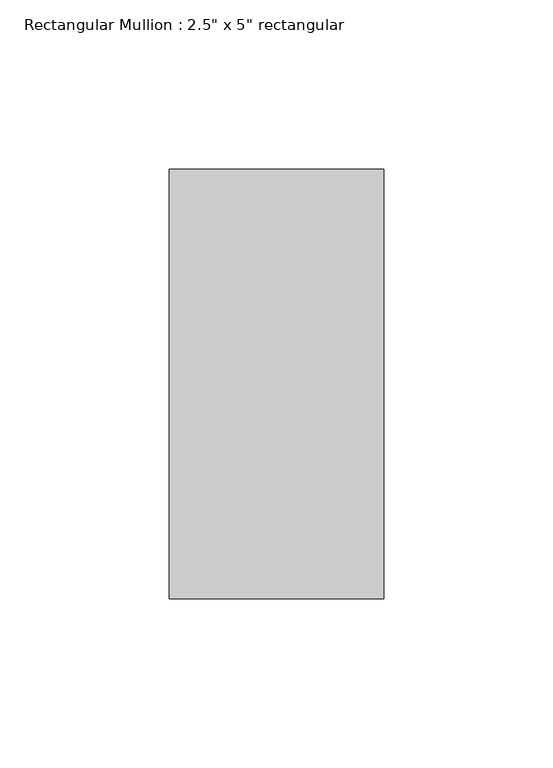
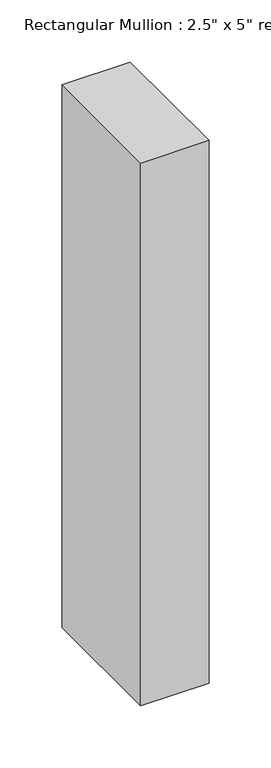
"""IFC4 building model written with IfcOpenShell, lengths in millimetres: member geometry."""

from ifc_helpers import new_model, si_unit, frame, origin, place, context, project, spatial, polyline, outline, extrude, source, transform, mapped, element, save


def member_b281fab0(model_context):
    return source(origin(), model_context, "Body", "SweptSolid", [
        extrude(outline(polyline([(0.0, 63.5), (0.0, -63.5), (-63.5, -63.5), (-63.5, 63.5), (0.0, 63.5)])), frame((0.0, 0.0, -533.4), z_axis=(0.0, 0.0, 1.0), x_axis=(1.0, 0.0, 0.0)), (0.0, 0.0, 1.0), 533.4),
    ])


if __name__ == "__main__":
    model = new_model("IFC4")
    model_context = context("Model", 3, world=origin())
    ifc_project = project(units=[si_unit("LENGTHUNIT", "METRE", prefix="MILLI")], contexts=[model_context])
    site = spatial("IfcSite", under=ifc_project)
    building = spatial("IfcBuilding", under=site)
    placement = place(None, origin())
    member_shape = member_b281fab0(model_context)
    element("IfcMember", 1, ObjectType="Rectangular Mullion : 2.5\" x 5\" rectangular", at=placement, inside=building, context=model_context, shape_type="MappedRepresentation", body=[
        mapped(member_shape, transform((0.0, 0.0, 0.0), x_axis=(1.0, 0.0, 0.0), y_axis=(0.0, 1.0, 0.0), z_axis=(0.0, 0.0, 1.0))),
    ])
    save(model, "model.ifc")

# Revit data of these elements
# Type "Rectangular Mullion : 2.5\" x 5\" rectangular"
#   built-in parameter 1007304 = 0.416667 (stored number, unit not read)
#   built-in parameter 1007301 = 0.104167 (stored number, unit not read)
#   built-in parameter 1007300 = 0.104167 (stored number, unit not read)
# Element 1 (IfcMember, "Rectangular Mullion : 2.5\" x 5\" rectangular")
#   Materials on its faces: "door colour"
# Materials
#   "door colour": class "Generic", colour RGB 120 120 120, transparency 0, Cost = 0
